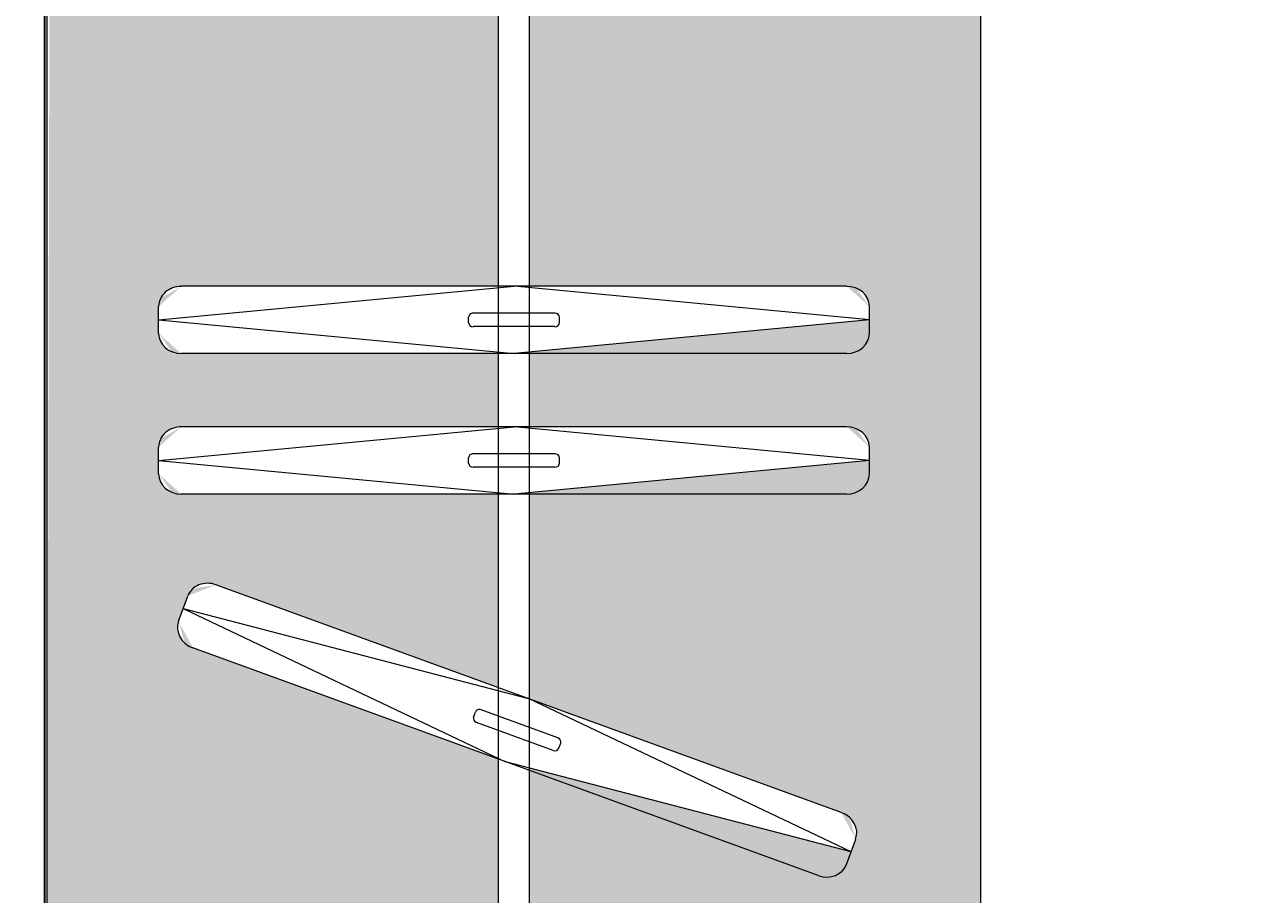
# Model space of a CAD drawing. Units: millimetres. Extents: x 27017497 to 27018854, y 7058029 to 7059154.
# Tile 6 of 91: x 27017622 to 27017651, y 7058146 to 7058166. Entities that reach past the tile are written whole.
import ezdxf

# ---------------------------------------------------------------- set-up
doc = ezdxf.new("R2010")
doc.units = ezdxf.units.MM
for name, color, linetype, lineweight in [('A-ANNO-DIMS', 2, 'Continuous', 18), ('A-FLOR-CASE', 8, 'Continuous', 20), ('A-FLOR-CASE-PATT', 44, 'Continuous', 13), ('A-WALL', 7, 'Continuous', 35)]:
    doc.layers.add(name, color=color, linetype=linetype, lineweight=lineweight)
doc.styles.get("Standard").update_dxf_attribs({"font": 'arial.ttf'})
doc.dimstyles.get("Standard").update_dxf_attribs({"dimtxt": 0.18, "dimasz": 0.18, "dimexe": 0.18, "dimexo": 0.0625, "dimgap": 0.09, "dimtad": 0, "dimtih": 1, "dimtoh": 1, "dimdec": 4, "dimzin": 0, "dimdsep": 46, "dimtxsty": 'Standard', "dimcen": 0.09, "dimadec": 0, "dimazin": 0, "dimtfac": 1, "dimtdec": 4, "dimtofl": 0, "dimtmove": 0, "dimatfit": 3, "dimfxl": 1, "dimtolj": 1, "dimtzin": 0, "dimarcsym": 0})

# ---------------------------------------------------------------- blocks, each defined once
blk = doc.blocks.new('WARDROBE-HANGING')
for p, q in [((0, 21.737), (65.212, 21.737)), ((47.493, 19.153), (46.71, 10.877)), ((47.806, 19.153), (47.18, 19.153)), ((47.493, 19.153), (48.276, 10.877)), ((50.766, 19.153), (49.984, 10.877)), ((51.079, 19.153), (50.453, 19.153)), ((50.766, 19.153), (51.549, 10.877)), ((60.171, 18.619), (59.582, 18.833)), ((46.71, 18.624), (46.71, 3.13)), ((48.276, 18.624), (48.276, 3.13)), ((49.984, 18.624), (49.984, 3.13)), ((51.549, 18.624), (51.549, 3.13)), ((58.961, 18.497), (53.661, 3.937)), ((59.877, 18.726), (56.311, 11.217)), ((59.877, 18.726), (57.782, 10.682)), ((60.431, 17.962), (55.132, 3.402)), ((47.336, 11.828), (47.336, 9.927)), ((47.556, 11.934), (47.43, 11.934)), ((47.649, 11.828), (47.649, 9.927)), ((50.61, 11.828), (50.61, 9.927)), ((50.829, 11.934), (50.704, 11.934)), ((50.923, 11.828), (50.923, 9.927)), ((57.224, 11.896), (56.574, 10.11)), ((57.466, 11.921), (57.349, 11.964)), ((57.519, 11.789), (56.868, 10.002)), ((0, 11.231), (65.212, 11.231)), ((54.216, 3.173), (56.311, 11.217)), ((47.493, 2.602), (46.71, 10.877)), ((47.493, 2.602), (48.276, 10.877)), ((50.766, 2.602), (49.984, 10.877)), ((50.766, 2.602), (51.549, 10.877)), ((54.216, 3.173), (57.782, 10.682)), ((0, 10.506), (65.212, 10.506)), ((47.556, 9.821), (47.43, 9.821)), ((50.829, 9.821), (50.704, 9.821)), ((56.744, 9.935), (56.626, 9.978)), ((54.51, 3.066), (53.922, 3.28)), ((47.806, 2.602), (47.18, 2.602)), ((51.079, 2.602), (50.453, 2.602)), ((0, 0), (65.212, 0))]:
    blk.add_line(p, q)
for centre, major_axis, start_param, end_param in [((47.18, 18.624), (0, 0.528), 0, 1.570796), ((47.806, 18.624), (0, 0.528), 4.712389, 6.283185), ((50.453, 18.624), (0, 0.528), 0, 1.570796), ((51.079, 18.624), (0, 0.528), 4.712389, 6.283185), ((59.402, 18.336), (0.181, 0.496), 0, 1.570796), ((59.99, 18.122), (0.181, 0.496), -1.570796, 0), ((47.43, 11.828), (0, 0.106), 0, 1.570796), ((47.556, 11.828), (0, 0.106), -1.570796, 0), ((50.704, 11.828), (0, 0.106), 0, 1.570796), ((50.829, 11.828), (0, 0.106), -1.570796, 0), ((57.313, 11.864), (0.0361, 0.0993), 0, 1.570796), ((57.43, 11.821), (0.0361, 0.0993), 4.712389, 6.283185), ((56.662, 10.077), (0.0361, 0.0993), 1.570796, 3.141593), ((47.43, 9.927), (0, 0.106), 1.570796, 3.141593), ((47.556, 9.927), (0, 0.106), 3.141593, 4.712389), ((50.704, 9.927), (0, 0.106), 1.570796, 3.141593), ((50.829, 9.927), (0, 0.106), 3.141593, 4.712389), ((56.78, 10.035), (0.0361, 0.0993), 3.141593, 4.712389), ((54.102, 3.777), (0.181, 0.496), 1.570796, 3.141593), ((54.691, 3.562), (0.181, 0.496), 3.141593, 4.712389), ((47.18, 3.13), (0, 0.528), 1.570796, 3.141593), ((47.806, 3.13), (0, 0.528), 3.141593, 4.712389), ((50.453, 3.13), (0, 0.528), 1.570796, 3.141593), ((51.079, 3.13), (0, 0.528), 3.141593, 4.712389)]:
    blk.add_ellipse(centre, major_axis=major_axis, ratio=0.888892, start_param=start_param, end_param=end_param)
blk = doc.blocks.new('*D47')
at = {"layer": 'A-ANNO-DIMS', "color": 0, "lineweight": -2, "transparency": 16777216}
for p, q in [((27017561.166, 7058294.35), (27017561.166, 7058028.6)), ((27018790.606, 7058294.35), (27018790.606, 7058028.6)), ((27017561.346, 7058028.78), (27018175.431, 7058028.78)), ((27018790.426, 7058028.78), (27018176.341, 7058028.78))]:
    blk.add_line(p, q, dxfattribs=at)
at = {"layer": 'A-ANNO-DIMS', "color": 0, "transparency": 16777216}
for points in [[(27017561.346, 7058028.81), (27017561.346, 7058028.75), (27017561.166, 7058028.78)], [(27018790.426, 7058028.81), (27018790.426, 7058028.75), (27018790.606, 7058028.78)]]:
    blk.add_solid(points, dxfattribs=at)
at = {"layer": 'Defpoints', "color": 0, "transparency": 16777216}
for p in [(27017561.166, 7058294.412), (27018790.606, 7058294.412), (27018790.606, 7058028.78)]:
    blk.add_point(p, dxfattribs=at)
at = {"layer": 'A-ANNO-DIMS', "color": 0, "transparency": 16777216, "insert": (27018175.886, 7058028.78), "char_height": 0.18, "attachment_point": 5}
blk.add_mtext('\\A1;1229.4', dxfattribs=at)
blk = doc.blocks.new('*D48')
at = {"layer": 'A-ANNO-DIMS', "color": 0, "lineweight": -2, "transparency": 16777216}
for p, q in [((27018463.498, 7058622.912), (27017497.536, 7058622.912)), ((27017497.716, 7058622.732), (27017497.716, 7058357.753)), ((27017497.716, 7058092.41), (27017497.716, 7058357.389)), ((27018555.129, 7058092.23), (27017497.536, 7058092.23))]:
    blk.add_line(p, q, dxfattribs=at)
at = {"layer": 'A-ANNO-DIMS', "color": 0, "transparency": 16777216}
for points in [[(27017497.686, 7058622.732), (27017497.746, 7058622.732), (27017497.716, 7058622.912)], [(27017497.686, 7058092.41), (27017497.746, 7058092.41), (27017497.716, 7058092.23)]]:
    blk.add_solid(points, dxfattribs=at)
at = {"layer": 'Defpoints', "color": 0, "transparency": 16777216}
for p in [(27018463.561, 7058622.912), (27017497.716, 7058092.23), (27018555.192, 7058092.23)]:
    blk.add_point(p, dxfattribs=at)
at = {"layer": 'A-ANNO-DIMS', "color": 0, "transparency": 16777216, "insert": (27017497.716, 7058357.571), "char_height": 0.18, "attachment_point": 5}
blk.add_mtext('\\A1;530.7', dxfattribs=at)

msp = doc.modelspace()

# ---------------------------------------------------------------- hatches: boundary and pattern name
at = {"layer": 'A-FLOR-CASE-PATT'}
h = msp.add_hatch(color=256, dxfattribs=at)
h.dxf.hatch_style = 1
edge = h.paths.add_edge_path()
edge.add_line((27017644.461, 7058207.1), (27017639.716, 7058207.1))
edge.add_line((27017639.716, 7058207.1), (27017639.716, 7058207.055))
edge.add_line((27017639.716, 7058207.055), (27017633.955, 7058207.055))
edge.add_line((27017633.955, 7058207.055), (27017633.955, 7058203.02))
edge.add_line((27017633.955, 7058203.02), (27017641.542, 7058203.02))
edge.add_ellipse((27017641.349, 7058202.551), major_axis=(0.528, 0), ratio=0.888892, start_angle=0, end_angle=90, ccw=False)
edge.add_line((27017641.877, 7058202.551), (27017641.877, 7058202.238))
edge.add_line((27017641.877, 7058202.238), (27017633.955, 7058201.488))
edge.add_line((27017633.955, 7058201.488), (27017633.955, 7058199.747))
edge.add_line((27017633.955, 7058199.747), (27017641.542, 7058199.747))
edge.add_ellipse((27017641.349, 7058199.277), major_axis=(0.528, 0), ratio=0.888892, start_angle=0, end_angle=90, ccw=False)
edge.add_line((27017641.877, 7058199.277), (27017641.877, 7058198.964))
edge.add_line((27017641.877, 7058198.964), (27017633.955, 7058198.215))
edge.add_line((27017633.955, 7058198.215), (27017633.955, 7058193.415))
edge.add_line((27017633.955, 7058193.415), (27017641.403, 7058190.704))
edge.add_ellipse((27017641.06, 7058190.329), major_axis=(0.496, -0.181), ratio=0.888892, start_angle=0, end_angle=90, ccw=False)
edge.add_line((27017641.557, 7058190.148), (27017641.45, 7058189.854))
edge.add_line((27017641.45, 7058189.854), (27017633.955, 7058191.806))
edge.add_line((27017633.955, 7058191.806), (27017633.955, 7058188.22))
edge.add_line((27017633.955, 7058188.22), (27017641.542, 7058188.22))
edge.add_ellipse((27017641.349, 7058187.75), major_axis=(0.528, 0), ratio=0.888892, start_angle=0, end_angle=90, ccw=False)
edge.add_line((27017641.877, 7058187.75), (27017641.877, 7058187.437))
edge.add_line((27017641.877, 7058187.437), (27017633.955, 7058186.688))
edge.add_line((27017633.955, 7058186.688), (27017633.955, 7058181.982))
edge.add_line((27017633.955, 7058181.982), (27017641.542, 7058181.982))
edge.add_ellipse((27017641.349, 7058181.513), major_axis=(0.528, 0), ratio=0.888892, start_angle=0, end_angle=90, ccw=False)
edge.add_line((27017641.877, 7058181.513), (27017641.877, 7058181.199))
edge.add_line((27017641.877, 7058181.199), (27017633.955, 7058180.45))
edge.add_line((27017633.955, 7058180.45), (27017633.955, 7058178.709))
edge.add_line((27017633.955, 7058178.709), (27017641.542, 7058178.709))
edge.add_ellipse((27017641.349, 7058178.239), major_axis=(0.528, 0), ratio=0.888892, start_angle=0, end_angle=90, ccw=False)
edge.add_line((27017641.877, 7058178.239), (27017641.877, 7058177.926))
edge.add_line((27017641.877, 7058177.926), (27017633.955, 7058177.177))
edge.add_line((27017633.955, 7058177.177), (27017633.955, 7058173.878))
edge.add_line((27017633.955, 7058173.878), (27017641.403, 7058171.167))
edge.add_ellipse((27017641.06, 7058170.792), major_axis=(0.496, -0.181), ratio=0.888892, start_angle=0, end_angle=90, ccw=False)
edge.add_line((27017641.557, 7058170.611), (27017641.45, 7058170.317))
edge.add_line((27017641.45, 7058170.317), (27017633.955, 7058172.269))
edge.add_line((27017633.955, 7058172.269), (27017633.955, 7058168.293))
edge.add_line((27017633.955, 7058168.293), (27017641.542, 7058168.293))
edge.add_ellipse((27017641.349, 7058167.824), major_axis=(0.528, 0), ratio=0.888892, start_angle=0, end_angle=90, ccw=False)
edge.add_line((27017641.877, 7058167.824), (27017641.877, 7058167.511))
edge.add_line((27017641.877, 7058167.511), (27017633.955, 7058166.762))
edge.add_line((27017633.955, 7058166.762), (27017633.955, 7058160.389))
edge.add_line((27017633.955, 7058160.389), (27017641.542, 7058160.389))
edge.add_ellipse((27017641.349, 7058159.92), major_axis=(0.528, 0), ratio=0.888892, start_angle=0, end_angle=90, ccw=False)
edge.add_line((27017641.877, 7058159.92), (27017641.877, 7058159.607))
edge.add_line((27017641.877, 7058159.607), (27017633.955, 7058158.858))
edge.add_line((27017633.955, 7058158.858), (27017633.955, 7058157.116))
edge.add_line((27017633.955, 7058157.116), (27017641.542, 7058157.116))
edge.add_ellipse((27017641.349, 7058156.647), major_axis=(0.528, 0), ratio=0.888892, start_angle=0, end_angle=90, ccw=False)
edge.add_line((27017641.877, 7058156.647), (27017641.877, 7058156.334))
edge.add_line((27017641.877, 7058156.334), (27017633.955, 7058155.585))
edge.add_line((27017633.955, 7058155.585), (27017633.955, 7058150.784))
edge.add_line((27017633.955, 7058150.784), (27017641.403, 7058148.073))
edge.add_ellipse((27017641.06, 7058147.698), major_axis=(0.496, -0.181), ratio=0.888892, start_angle=0, end_angle=90, ccw=False)
edge.add_line((27017641.557, 7058147.517), (27017641.45, 7058147.223))
edge.add_line((27017641.45, 7058147.223), (27017633.955, 7058149.175))
edge.add_line((27017633.955, 7058149.175), (27017633.955, 7058145.589))
edge.add_line((27017633.955, 7058145.589), (27017641.542, 7058145.589))
edge.add_ellipse((27017641.349, 7058145.119), major_axis=(0.528, 0), ratio=0.888892, start_angle=0, end_angle=90, ccw=False)
edge.add_line((27017641.877, 7058145.119), (27017641.877, 7058144.806))
edge.add_line((27017641.877, 7058144.806), (27017633.955, 7058144.057))
edge.add_line((27017633.955, 7058144.057), (27017633.955, 7058141.912))
edge.add_line((27017633.955, 7058141.912), (27017644.461, 7058141.912))
edge.add_line((27017644.461, 7058141.912), (27017644.461, 7058207.1))
edge = h.paths.add_edge_path()
edge.add_ellipse((27017626.287, 7058195.04), major_axis=(0.496, -0.181), ratio=0.888892, start_angle=180, end_angle=270, ccw=False)
edge.add_line((27017625.79, 7058195.22), (27017626.063, 7058195.97))
edge.add_ellipse((27017626.501, 7058195.628), major_axis=(0.496, -0.181), ratio=0.888892, start_angle=90, end_angle=180, ccw=False)
edge.add_line((27017626.661, 7058196.069), (27017633.23, 7058193.678))
edge.add_line((27017633.23, 7058193.678), (27017633.23, 7058198.182))
edge.add_line((27017633.23, 7058198.182), (27017625.661, 7058198.182))
edge.add_ellipse((27017625.854, 7058198.651), major_axis=(0.528, 0), ratio=0.888892, start_angle=180, end_angle=270, ccw=False)
edge.add_line((27017625.326, 7058198.651), (27017625.326, 7058199.449))
edge.add_ellipse((27017625.854, 7058199.277), major_axis=(0.528, 0), ratio=0.888892, start_angle=90, end_angle=180, ccw=False)
edge.add_line((27017625.854, 7058199.747), (27017633.23, 7058199.747))
edge.add_line((27017633.23, 7058199.747), (27017633.23, 7058201.455))
edge.add_line((27017633.23, 7058201.455), (27017625.661, 7058201.455))
edge.add_ellipse((27017625.854, 7058201.924), major_axis=(0.528, 0), ratio=0.888892, start_angle=180, end_angle=270, ccw=False)
edge.add_line((27017625.326, 7058201.924), (27017625.326, 7058202.722))
edge.add_ellipse((27017625.854, 7058202.551), major_axis=(0.528, 0), ratio=0.888892, start_angle=90, end_angle=180, ccw=False)
edge.add_line((27017625.854, 7058203.02), (27017633.23, 7058203.02))
edge.add_line((27017633.23, 7058203.02), (27017633.23, 7058207.055))
edge.add_line((27017633.23, 7058207.055), (27017622.865, 7058207.055))
edge.add_line((27017622.865, 7058207.055), (27017622.865, 7058201.7))
edge.add_line((27017622.865, 7058201.7), (27017622.724, 7058141.912))
edge.add_line((27017622.724, 7058141.912), (27017633.23, 7058141.912))
edge.add_line((27017633.23, 7058141.912), (27017633.23, 7058144.024))
edge.add_line((27017633.23, 7058144.024), (27017625.661, 7058144.024))
edge.add_ellipse((27017625.854, 7058144.493), major_axis=(0.528, 0), ratio=0.888892, start_angle=180, end_angle=270, ccw=False)
edge.add_line((27017625.326, 7058144.493), (27017625.326, 7058145.291))
edge.add_ellipse((27017625.854, 7058145.119), major_axis=(0.528, 0), ratio=0.888892, start_angle=90, end_angle=180, ccw=False)
edge.add_line((27017625.854, 7058145.589), (27017633.23, 7058145.589))
edge.add_line((27017633.23, 7058145.589), (27017633.23, 7058149.382))
edge.add_line((27017633.23, 7058149.382), (27017625.944, 7058152.034))
edge.add_ellipse((27017626.287, 7058152.409), major_axis=(0.496, -0.181), ratio=0.888892, start_angle=180, end_angle=270, ccw=False)
edge.add_line((27017625.79, 7058152.59), (27017626.063, 7058153.34))
edge.add_ellipse((27017626.501, 7058152.997), major_axis=(0.496, -0.181), ratio=0.888892, start_angle=90, end_angle=180, ccw=False)
edge.add_line((27017626.661, 7058153.439), (27017633.23, 7058151.048))
edge.add_line((27017633.23, 7058151.048), (27017633.23, 7058155.551))
edge.add_line((27017633.23, 7058155.551), (27017625.661, 7058155.551))
edge.add_ellipse((27017625.854, 7058156.021), major_axis=(0.528, 0), ratio=0.888892, start_angle=180, end_angle=270, ccw=False)
edge.add_line((27017625.326, 7058156.021), (27017625.326, 7058156.819))
edge.add_ellipse((27017625.854, 7058156.647), major_axis=(0.528, 0), ratio=0.888892, start_angle=90, end_angle=180, ccw=False)
edge.add_line((27017625.854, 7058157.116), (27017633.23, 7058157.116))
edge.add_line((27017633.23, 7058157.116), (27017633.23, 7058158.824))
edge.add_line((27017633.23, 7058158.824), (27017625.661, 7058158.824))
edge.add_ellipse((27017625.854, 7058159.294), major_axis=(0.528, 0), ratio=0.888892, start_angle=180, end_angle=270, ccw=False)
edge.add_line((27017625.326, 7058159.294), (27017625.326, 7058160.092))
edge.add_ellipse((27017625.854, 7058159.92), major_axis=(0.528, 0), ratio=0.888892, start_angle=90, end_angle=180, ccw=False)
edge.add_line((27017625.854, 7058160.389), (27017633.23, 7058160.389))
edge.add_line((27017633.23, 7058160.389), (27017633.23, 7058166.728))
edge.add_line((27017633.23, 7058166.728), (27017625.661, 7058166.728))
edge.add_ellipse((27017625.854, 7058167.198), major_axis=(0.528, 0), ratio=0.888892, start_angle=180, end_angle=270, ccw=False)
edge.add_line((27017625.326, 7058167.198), (27017625.326, 7058167.996))
edge.add_ellipse((27017625.854, 7058167.824), major_axis=(0.528, 0), ratio=0.888892, start_angle=90, end_angle=180, ccw=False)
edge.add_line((27017625.854, 7058168.293), (27017633.23, 7058168.293))
edge.add_line((27017633.23, 7058168.293), (27017633.23, 7058172.476))
edge.add_line((27017633.23, 7058172.476), (27017625.944, 7058175.128))
edge.add_ellipse((27017626.287, 7058175.503), major_axis=(0.496, -0.181), ratio=0.888892, start_angle=180, end_angle=270, ccw=False)
edge.add_line((27017625.79, 7058175.684), (27017626.063, 7058176.433))
edge.add_ellipse((27017626.501, 7058176.091), major_axis=(0.496, -0.181), ratio=0.888892, start_angle=90, end_angle=180, ccw=False)
edge.add_line((27017626.661, 7058176.533), (27017633.23, 7058174.142))
edge.add_line((27017633.23, 7058174.142), (27017633.23, 7058177.144))
edge.add_line((27017633.23, 7058177.144), (27017625.661, 7058177.144))
edge.add_ellipse((27017625.854, 7058177.613), major_axis=(0.528, 0), ratio=0.888892, start_angle=180, end_angle=270, ccw=False)
edge.add_line((27017625.326, 7058177.613), (27017625.326, 7058178.411))
edge.add_ellipse((27017625.854, 7058178.239), major_axis=(0.528, 0), ratio=0.888892, start_angle=90, end_angle=180, ccw=False)
edge.add_line((27017625.854, 7058178.709), (27017633.23, 7058178.709))
edge.add_line((27017633.23, 7058178.709), (27017633.23, 7058180.417))
edge.add_line((27017633.23, 7058180.417), (27017625.661, 7058180.417))
edge.add_ellipse((27017625.854, 7058180.886), major_axis=(0.528, 0), ratio=0.888892, start_angle=180, end_angle=270, ccw=False)
edge.add_line((27017625.326, 7058180.886), (27017625.326, 7058181.684))
edge.add_ellipse((27017625.854, 7058181.513), major_axis=(0.528, 0), ratio=0.888892, start_angle=90, end_angle=180, ccw=False)
edge.add_line((27017625.854, 7058181.982), (27017633.23, 7058181.982))
edge.add_line((27017633.23, 7058181.982), (27017633.23, 7058186.655))
edge.add_line((27017633.23, 7058186.655), (27017625.661, 7058186.655))
edge.add_ellipse((27017625.854, 7058187.124), major_axis=(0.528, 0), ratio=0.888892, start_angle=180, end_angle=270, ccw=False)
edge.add_line((27017625.326, 7058187.124), (27017625.326, 7058187.922))
edge.add_ellipse((27017625.854, 7058187.75), major_axis=(0.528, 0), ratio=0.888892, start_angle=90, end_angle=180, ccw=False)
edge.add_line((27017625.854, 7058188.22), (27017633.23, 7058188.22))
edge.add_line((27017633.23, 7058188.22), (27017633.23, 7058192.013))
edge.add_line((27017633.23, 7058192.013), (27017625.944, 7058194.665))

# ---------------------------------------------------------------- linework, layer by layer
at = {"layer": 'A-WALL'}
msp.add_line((27017622.666, 7058294.412), (27017622.666, 7058141.912), dxfattribs=at)

# ---------------------------------------------------------------- block references
at = {"layer": 'A-FLOR-CASE', "rotation": 270}
msp.add_blockref('WARDROBE-HANGING', (27017622.724, 7058207.1), dxfattribs=at)

# ---------------------------------------------------------------- dimensions: what is measured, and where the dimension line sits
at = {"layer": 'A-ANNO-DIMS'}
dim = msp.add_linear_dim(base=(27017497.716, 7058092.23), p1=(27018463.561, 7058622.912), p2=(27018555.192, 7058092.23), angle=90, dimstyle='Standard', override={"dimdec": 1, "dimlfac": 1, "dimrnd": 0, "dimzin": 0, "dimdsep": 46, "dimlunit": 2}, dxfattribs=at)
dim.commit()
dim.dimension.update_dxf_attribs({"geometry": '*D48', "text_midpoint": (27017497.716, 7058357.571)})
dim = msp.add_linear_dim(base=(27018790.606, 7058028.78), p1=(27017561.166, 7058294.412), p2=(27018790.606, 7058294.412), dimstyle='Standard', override={"dimdec": 1, "dimlfac": 1, "dimrnd": 0, "dimzin": 0, "dimdsep": 46, "dimlunit": 2}, dxfattribs=at)
dim.commit()
dim.dimension.update_dxf_attribs({"geometry": '*D47', "text_midpoint": (27018175.886, 7058028.78)})

doc.saveas('drawing.dxf')
